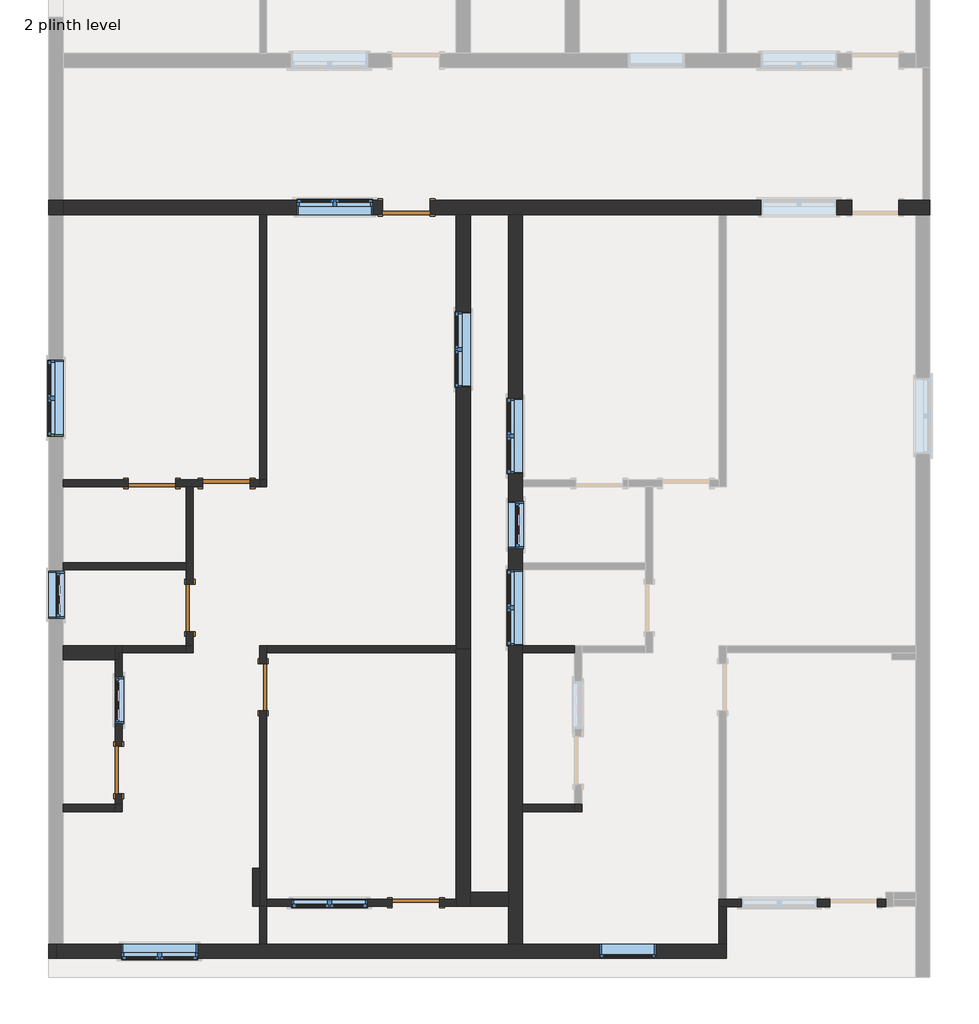
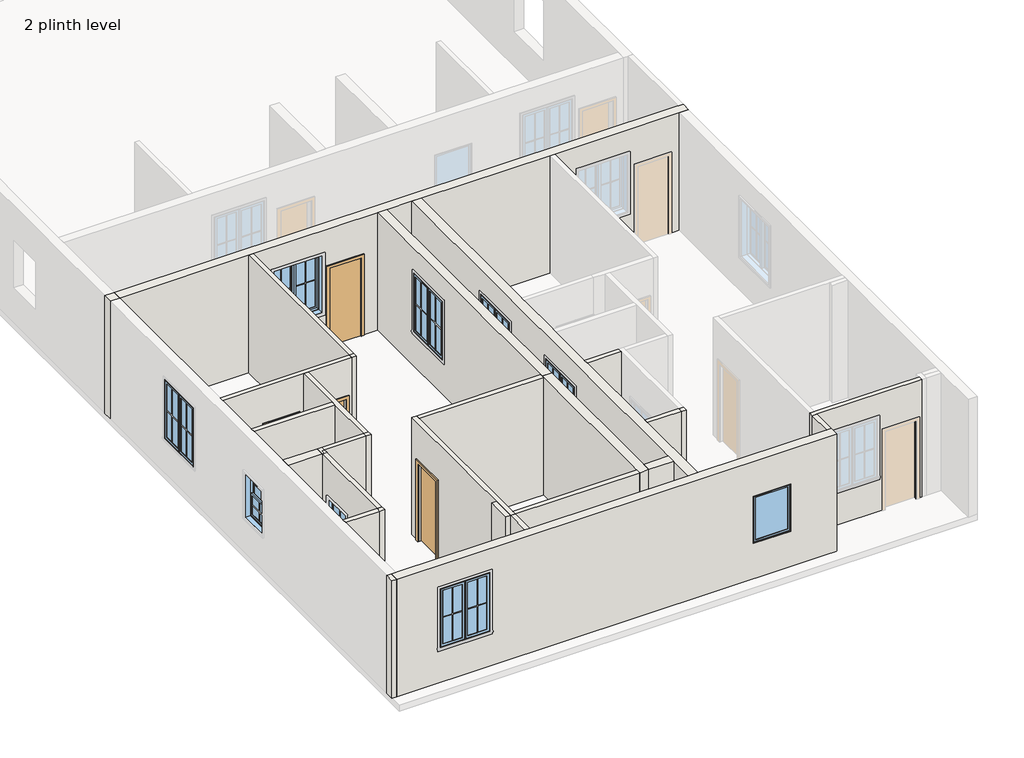
# One storey, part 1 of 4: 30 walls, 11 windows, 7 doors.
"""IFC4 building model written with IfcOpenShell, lengths in millimetres."""

from ifc_helpers import new_model, si_unit, frame, origin, place, context, project, spatial, polyline, outline, extrude, faceted_brep, transform, mapped, element, save
from components import door_d8f5dbb5, door_f2b275c1, door_85036156, window_c1f32544, window_8377141f, window_d9d3dda5, window_d400040f, window_5a369d27

model = new_model("IFC4")

# Units and contexts
model_context = context("Model", 3, world=origin())
ifc_project = project(units=[si_unit("LENGTHUNIT", "METRE", prefix="MILLI")], contexts=[model_context])

# Site, building, storey
site = spatial("IfcSite", under=ifc_project)
building = spatial("IfcBuilding", under=site)
storey = spatial("IfcBuildingStorey", under=building, Name="2 plinth level", Elevation=457.2)

# Doors
placement = place(None, origin())
door_shape = door_d8f5dbb5(model_context)
element("IfcDoor", 1, ObjectType="Single-Flush : 30\" x 80\"", at=placement, inside=storey, context=model_context, shape_type="MappedRepresentation", body=[
    mapped(door_shape, transform((-2447.3775468, -11601.0304449, 457.2), x_axis=(1.0, 0.0, 0.0), y_axis=(0.0, 1.0, 0.0), z_axis=(0.0, 0.0, 1.0))),
])
element("IfcDoor", 2, ObjectType="Single-Flush : 30\" x 80\"", at=placement, inside=storey, context=model_context, shape_type="MappedRepresentation", body=[
    mapped(door_shape, transform((-5495.3775468, -4857.3304449, 457.2), x_axis=(1.0, 0.0, 0.0), y_axis=(0.0, 1.0, 0.0), z_axis=(0.0, 0.0, 1.0))),
])
door_2_shape = door_f2b275c1(model_context)
element("IfcDoor", 3, ObjectType="Single-Flush : 30\" x 80\"", at=placement, inside=storey, context=model_context, shape_type="MappedRepresentation", body=[
    mapped(door_2_shape, transform((-4904.8275468, -8133.9304449, 457.2), x_axis=(0.0, 1.0, 0.0), y_axis=(-1.0, 0.0, 0.0), z_axis=(0.0, 0.0, 1.0))),
])
element("IfcDoor", 4, ObjectType="Single-Flush : 30\" x 80\"", at=placement, inside=storey, context=model_context, shape_type="MappedRepresentation", body=[
    mapped(door_2_shape, transform((-7228.9275468, -9467.4304449, 457.2), x_axis=(0.0, -1.0, 0.0), y_axis=(1.0, 0.0, 0.0), z_axis=(0.0, 0.0, 1.0))),
])
element("IfcDoor", 5, ObjectType="Single-Flush : 30\" x 80\"", at=placement, inside=storey, context=model_context, shape_type="MappedRepresentation", body=[
    mapped(door_2_shape, transform((-6085.9275468, -6857.5804449, 457.2), x_axis=(0.0, -1.0, 0.0), y_axis=(1.0, 0.0, 0.0), z_axis=(0.0, 0.0, 1.0))),
])
element("IfcDoor", 6, ObjectType="Single-Flush : 30\" x 80\"", at=placement, inside=storey, context=model_context, shape_type="MappedRepresentation", body=[
    mapped(door_2_shape, transform((-6695.5275468, -4857.3304449, 457.2), x_axis=(1.0, 0.0, 0.0), y_axis=(0.0, 1.0, 0.0), z_axis=(0.0, 0.0, 1.0))),
])
door_3_shape = door_85036156(model_context)
element("IfcDoor", 7, ObjectType="Single-Flush : 30\" x 80\"", at=placement, inside=storey, context=model_context, shape_type="MappedRepresentation", body=[
    mapped(door_3_shape, transform((-2599.7775468, -418.6804449, 457.2), x_axis=(1.0, 0.0, 0.0), y_axis=(0.0, 1.0, 0.0), z_axis=(0.0, 0.0, 1.0))),
])

# Walls
element("IfcWall", 8, ObjectType="4.5\"", at=placement, inside=storey, context=model_context, shape_type="Brep", body=[
    faceted_brep([(-5114.3775468, -4914.4804449, 2489.2), (-5114.3775468, -4914.4804449, 457.2), (-4961.9775468, -4914.4804449, 457.2), (-4961.9775468, -4914.4804449, 3505.2), (-6028.7775468, -4914.4804449, 3505.2), (-6143.0775468, -4914.4804449, 3505.2), (-8124.2775468, -4914.4804449, 3505.2), (-8124.2775468, -4914.4804449, 457.2), (-7076.5275468, -4914.4804449, 457.2), (-7076.5275468, -4914.4804449, 2489.2), (-6314.5275468, -4914.4804449, 2489.2), (-6314.5275468, -4914.4804449, 457.2), (-6143.0775468, -4914.4804449, 457.2), (-6028.7775468, -4914.4804449, 457.2), (-5876.3775468, -4914.4804449, 457.2), (-5876.3775468, -4914.4804449, 2489.2), (-4961.9775468, -4800.1804449, 457.2), (-5114.3775468, -4800.1804449, 457.2), (-5114.3775468, -4800.1804449, 2489.2), (-5876.3775468, -4800.1804449, 2489.2), (-5876.3775468, -4800.1804449, 457.2), (-6314.5275468, -4800.1804449, 457.2), (-6314.5275468, -4800.1804449, 2489.2), (-7076.5275468, -4800.1804449, 2489.2), (-7076.5275468, -4800.1804449, 457.2), (-8124.2775468, -4800.1804449, 457.2), (-8124.2775468, -4800.1804449, 3505.2), (-4961.9775468, -4800.1804449, 3505.2)], [[[0, 1, 2, 3, 4, 5, 6, 7, 8, 9, 10, 11, 12, 13, 14, 15]], [[16, 17, 18, 19, 20, 21, 22, 23, 24, 25, 26, 27]], [[8, 7, 25, 24]], [[2, 1, 17, 16]], [[14, 13, 12, 11, 21, 20]], [[6, 5, 4, 3, 27, 26]], [[7, 6, 26, 25]], [[3, 2, 16, 27]], [[22, 21, 11, 10]], [[23, 22, 10, 9]], [[24, 23, 9, 8]], [[18, 17, 1, 0]], [[19, 18, 0, 15]], [[20, 19, 15, 14]]]),
])
element("IfcWall", 9, ObjectType="4.5\"", at=placement, inside=storey, context=model_context, shape_type="Brep", body=[
    faceted_brep([(-6028.7775468, -7467.1804449, 457.2), (-6028.7775468, -7238.5804449, 457.2), (-6028.7775468, -7238.5804449, 2489.2), (-6028.7775468, -6476.5804449, 2489.2), (-6028.7775468, -6476.5804449, 457.2), (-6028.7775468, -4914.4804449, 457.2), (-6028.7775468, -4914.4804449, 3505.2), (-6028.7775468, -7467.1804449, 3505.2), (-6143.0775468, -7238.5804449, 2489.2), (-6143.0775468, -7238.5804449, 457.2), (-6143.0775468, -7467.1804449, 457.2), (-6143.0775468, -7467.1804449, 3505.2), (-6143.0775468, -6247.9804448, 3505.2), (-6143.0775468, -6133.6804448, 3505.2), (-6143.0775468, -4914.4804449, 3505.2), (-6143.0775468, -4914.4804449, 457.2), (-6143.0775468, -6133.6804448, 457.2), (-6143.0775468, -6247.9804448, 457.2), (-6143.0775468, -6476.5804449, 457.2), (-6143.0775468, -6476.5804449, 2489.2)], [[[0, 1, 2, 3, 4, 5, 6, 7]], [[8, 9, 10, 11, 12, 13, 14, 15, 16, 17, 18, 19]], [[10, 9, 1, 0]], [[18, 17, 16, 15, 5, 4]], [[7, 6, 14, 13, 12, 11]], [[0, 7, 11, 10]], [[6, 5, 15, 14]], [[2, 1, 9, 8]], [[3, 2, 8, 19]], [[4, 3, 19, 18]]]),
])
element("IfcWall", 10, ObjectType="4.5\"", at=placement, inside=storey, context=model_context, shape_type="SweptSolid", body=[
    extrude(outline(polyline([(-4847.6775468, -4800.1804449), (-4847.6775468, -4914.4804449), (-4961.9775468, -4914.4804449), (-4961.9775468, -4800.1804449), (-4847.6775468, -4800.1804449)])), frame((0.0, 0.0, 457.2), z_axis=(0.0, 0.0, 1.0), x_axis=(1.0, 0.0, 0.0)), (0.0, 0.0, 1.0), 3048.0),
])
element("IfcWall", 11, ObjectType="4.5\"", at=placement, inside=storey, context=model_context, shape_type="Brep", body=[
    faceted_brep([(-4847.6775468, -7752.9304449, 2489.2), (-4847.6775468, -7752.9304449, 457.2), (-4847.6775468, -7581.4804449, 457.2), (-4847.6775468, -7467.1804449, 457.2), (-4847.6775468, -7467.1804449, 3505.2), (-4847.6775468, -7581.4804449, 3505.2), (-4847.6775468, -11543.8804449, 3505.2), (-4847.6775468, -11658.1804449, 3505.2), (-4847.6775468, -11658.1804449, 457.2), (-4847.6775468, -11543.8804449, 457.2), (-4847.6775468, -8514.9304449, 457.2), (-4847.6775468, -8514.9304449, 2489.2), (-4961.9775468, -7467.1804449, 457.2), (-4961.9775468, -7752.9304449, 457.2), (-4961.9775468, -7752.9304449, 2489.2), (-4961.9775468, -8514.9304449, 2489.2), (-4961.9775468, -8514.9304449, 457.2), (-4961.9775468, -11658.1804449, 457.2), (-4961.9775468, -11658.1804449, 3505.2), (-4961.9775468, -7467.1804449, 3505.2)], [[[0, 1, 2, 3, 4, 5, 6, 7, 8, 9, 10, 11]], [[12, 13, 14, 15, 16, 17, 18, 19]], [[10, 9, 8, 17, 16]], [[3, 2, 1, 13, 12]], [[7, 6, 5, 4, 19, 18]], [[8, 7, 18, 17]], [[4, 3, 12, 19]], [[14, 13, 1, 0]], [[15, 14, 0, 11]], [[16, 15, 11, 10]]]),
])
element("IfcWall", 12, ObjectType="4.5\"", at=placement, inside=storey, context=model_context, shape_type="Brep", body=[
    faceted_brep([(-2066.3775468, -11658.1804449, 2489.2), (-2066.3775468, -11658.1804449, 457.2), (-1799.6775468, -11658.1804449, 457.2), (-1799.6775468, -11658.1804449, 3505.2), (-4847.6775468, -11658.1804449, 3505.2), (-4847.6775468, -11658.1804449, 457.2), (-2828.3775468, -11658.1804449, 457.2), (-2828.3775468, -11658.1804449, 2489.2), (-4447.6275468, -11658.1804449, 2895.6), (-3228.4275468, -11658.1804449, 2895.6), (-3228.4275468, -11658.1804449, 1371.6), (-4447.6275468, -11658.1804449, 1371.6), (-1799.6775468, -11543.8804449, 457.2), (-2066.3775468, -11543.8804449, 457.2), (-2066.3775468, -11543.8804449, 2489.2), (-2828.3775468, -11543.8804449, 2489.2), (-2828.3775468, -11543.8804449, 457.2), (-4847.6775468, -11543.8804449, 457.2), (-4847.6775468, -11543.8804449, 3505.2), (-1799.6775468, -11543.8804449, 3505.2), (-4447.6275468, -11543.8804449, 2895.6), (-4447.6275468, -11543.8804449, 1371.6), (-3228.4275468, -11543.8804449, 1371.6), (-3228.4275468, -11543.8804449, 2895.6), (-1799.6775468, -11657.3545138, 457.2), (-1799.6775468, -11657.3545138, 3505.2)], [[[0, 1, 2, 3, 4, 5, 6, 7], [8, 9, 10, 11]], [[12, 13, 14, 15, 16, 17, 18, 19], [20, 21, 22, 23]], [[6, 5, 17, 16]], [[2, 1, 13, 12, 24]], [[4, 3, 25, 19, 18]], [[5, 4, 18, 17]], [[3, 2, 24, 12, 19, 25]], [[14, 13, 1, 0]], [[15, 14, 0, 7]], [[16, 15, 7, 6]], [[21, 20, 8, 11]], [[22, 21, 11, 10]], [[23, 22, 10, 9]], [[20, 23, 9, 8]]]),
])
element("IfcWall", 13, ObjectType="4.5\"", at=placement, inside=storey, context=model_context, shape_type="SweptSolid", body=[
    extrude(outline(polyline([(-7171.7775468, -10134.1804449), (-7286.0775468, -10134.1804449), (-7286.0775468, -10019.8804449), (-7171.7775468, -10019.8804449), (-7171.7775468, -10134.1804449)])), frame((0.0, 0.0, 457.2), z_axis=(0.0, 0.0, 1.0), x_axis=(1.0, 0.0, 0.0)), (0.0, 0.0, 1.0), 3048.0),
])
element("IfcWall", 14, ObjectType="4.5\"", at=placement, inside=storey, context=model_context, shape_type="Brep", body=[
    faceted_brep([(-7286.0775468, -7467.1804449, 457.2), (-7286.0775468, -7695.7804449, 457.2), (-7286.0775468, -7695.7804449, 3505.2), (-7286.0775468, -7467.1804449, 3505.2), (-7171.7775468, -7467.1804449, 457.2), (-7171.7775468, -7467.1804449, 3505.2), (-7171.7775468, -7581.4804449, 3505.2), (-7171.7775468, -7695.7804449, 3505.2), (-7171.7775468, -7695.7804449, 457.2), (-7171.7775468, -7581.4804449, 457.2)], [[[0, 1, 2, 3]], [[4, 5, 6, 7, 8, 9]], [[1, 0, 4, 9, 8]], [[2, 1, 8, 7]], [[3, 2, 7, 6, 5]], [[0, 3, 5, 4]]]),
])
element("IfcWall", 15, ObjectType="4.5\"", at=placement, inside=storey, context=model_context, shape_type="SweptSolid", body=[
    extrude(outline(polyline([(-8124.2775468, -6133.6804448), (-6143.0775468, -6133.6804448), (-6143.0775468, -6247.9804448), (-8124.2775468, -6247.9804448), (-8124.2775468, -6133.6804448)])), frame((0.0, 0.0, 457.2), z_axis=(0.0, 0.0, 1.0), x_axis=(1.0, 0.0, 0.0)), (0.0, 0.0, 1.0), 3048.0),
])
element("IfcWall", 16, ObjectType="4.5\"", at=placement, inside=storey, context=model_context, shape_type="Brep", body=[
    faceted_brep([(-7171.7775468, -10019.8804449, 457.2), (-7171.7775468, -9848.4304449, 457.2), (-7171.7775468, -9848.4304449, 2489.2), (-7171.7775468, -9086.4304449, 2489.2), (-7171.7775468, -9086.4304449, 457.2), (-7171.7775468, -7581.4804449, 457.2), (-7171.7775468, -7581.4804449, 3505.2), (-7171.7775468, -10019.8804449, 3505.2), (-7171.7775468, -7962.4804449, 2540.0), (-7171.7775468, -7962.4804449, 1371.6), (-7171.7775468, -8724.4804449, 1371.6), (-7171.7775468, -8724.4804449, 2540.0), (-7286.0775468, -9848.4304449, 2489.2), (-7286.0775468, -9848.4304449, 457.2), (-7286.0775468, -10019.8804449, 457.2), (-7286.0775468, -10019.8804449, 3505.2), (-7286.0775468, -7695.7804449, 3505.2), (-7286.0775468, -7695.7804449, 457.2), (-7286.0775468, -9086.4304449, 457.2), (-7286.0775468, -9086.4304449, 2489.2), (-7286.0775468, -7962.4804449, 2540.0), (-7286.0775468, -8724.4804449, 2540.0), (-7286.0775468, -8724.4804449, 1371.6), (-7286.0775468, -7962.4804449, 1371.6), (-7228.9275468, -7695.7804449, 457.2), (-7228.9275468, -7581.4804449, 457.2), (-7228.9275468, -7581.4804449, 3505.2), (-7228.9275468, -7695.7804449, 3505.2)], [[[0, 1, 2, 3, 4, 5, 6, 7], [8, 9, 10, 11]], [[12, 13, 14, 15, 16, 17, 18, 19], [20, 21, 22, 23]], [[18, 17, 24, 25, 5, 4]], [[14, 13, 1, 0]], [[7, 6, 26, 27, 16, 15]], [[6, 5, 25, 26]], [[25, 24, 27, 26]], [[24, 17, 16, 27]], [[0, 7, 15, 14]], [[2, 1, 13, 12]], [[3, 2, 12, 19]], [[4, 3, 19, 18]], [[9, 8, 20, 23]], [[10, 9, 23, 22]], [[11, 10, 22, 21]], [[8, 11, 21, 20]]]),
])
element("IfcWall", 17, ObjectType="4.5\"", at=placement, inside=storey, context=model_context, shape_type="SweptSolid", body=[
    extrude(outline(polyline([(-6028.7775468, -7581.4804449), (-6143.0775468, -7581.4804449), (-6143.0775468, -7467.1804449), (-6028.7775468, -7467.1804449), (-6028.7775468, -7581.4804449)])), frame((0.0, 0.0, 457.2), z_axis=(0.0, 0.0, 1.0), x_axis=(1.0, 0.0, 0.0)), (0.0, 0.0, 1.0), 3048.0),
])
element("IfcWall", 18, ObjectType="4.5\"", at=placement, inside=storey, context=model_context, shape_type="SweptSolid", body=[
    extrude(outline(polyline([(-4961.9775468, -12267.7804449), (-4961.9775468, -11658.1804449), (-4847.6775468, -11658.1804449), (-4847.6775468, -12267.7804449), (-4961.9775468, -12267.7804449)])), frame((0.0, 0.0, 457.2), z_axis=(0.0, 0.0, 1.0), x_axis=(1.0, 0.0, 0.0)), (0.0, 0.0, 1.0), 3048.0),
])
element("IfcWall", 19, ObjectType="4.5\"", at=placement, inside=storey, context=model_context, shape_type="Brep", body=[
    faceted_brep([(5114.9115487, -11546.9284449, 457.2), (4971.996455, -11546.9284449, 457.2), (4971.996455, -11546.9284449, 2489.2), (4209.996455, -11546.9284449, 2489.2), (4209.996455, -11546.9284449, 457.2), (4067.0813613, -11546.9284449, 457.2), (3952.7813613, -11546.9284449, 457.2), (2543.7224532, -11546.9284449, 457.2), (2429.4224532, -11546.9284449, 457.2), (2429.4224532, -11546.9284449, 3505.2), (2543.7224532, -11546.9284449, 3505.2), (3952.7813613, -11546.9284449, 3505.2), (4067.0813613, -11546.9284449, 3505.2), (5114.9115487, -11546.9284449, 3505.2), (2790.7313613, -11546.9284449, 2895.6), (2790.7313613, -11546.9284449, 1371.6), (4009.9313613, -11546.9284449, 1371.6), (4009.9313613, -11546.9284449, 2895.6), (4971.996455, -11661.2284449, 2489.2), (4971.996455, -11661.2284449, 457.2), (5114.9115487, -11661.2284449, 457.2), (5114.9115487, -11661.2284449, 3505.2), (2543.7224532, -11661.2284449, 3505.2), (2429.4224532, -11661.2284449, 3505.2), (2429.4224532, -11661.2284449, 457.2), (2543.7224532, -11661.2284449, 457.2), (4209.996455, -11661.2284449, 457.2), (4209.996455, -11661.2284449, 2489.2), (2790.7313613, -11661.2284449, 2895.6), (4009.9313613, -11661.2284449, 2895.6), (4009.9313613, -11661.2284449, 1371.6), (2790.7313613, -11661.2284449, 1371.6)], [[[0, 1, 2, 3, 4, 5, 6, 7, 8, 9, 10, 11, 12, 13], [14, 15, 16, 17]], [[18, 19, 20, 21, 22, 23, 24, 25, 26, 27], [28, 29, 30, 31]], [[20, 19, 1, 0]], [[26, 25, 24, 8, 7, 6, 5, 4]], [[13, 12, 11, 10, 9, 23, 22, 21]], [[9, 8, 24, 23]], [[0, 13, 21, 20]], [[2, 1, 19, 18]], [[3, 2, 18, 27]], [[4, 3, 27, 26]], [[15, 14, 28, 31]], [[16, 15, 31, 30]], [[17, 16, 30, 29]], [[14, 17, 29, 28]]]),
])
element("IfcWall", 20, ObjectType="4.5\"", at=placement, inside=storey, context=model_context, shape_type="Brep", body=[
    faceted_brep([(-4847.6775468, -7581.4804449, 457.2), (-1799.6775468, -7581.4804449, 457.2), (-1799.6775468, -7581.4804449, 3505.2), (-4847.6775468, -7581.4804449, 3505.2), (-4847.6775468, -7467.1804449, 457.2), (-4847.6775468, -7467.1804449, 3505.2), (-1799.6775468, -7467.1804449, 3505.2), (-1799.6775468, -7467.1804449, 457.2), (-1799.6775468, -7524.3304449, 457.2), (-1799.6775468, -7524.3304449, 3505.2)], [[[0, 1, 2, 3]], [[4, 5, 6, 7]], [[1, 0, 4, 7, 8]], [[3, 2, 9, 6, 5]], [[2, 1, 8, 7, 6, 9]], [[0, 3, 5, 4]]]),
])
element("IfcWall", 21, ObjectType="4.5\"", at=placement, inside=storey, context=model_context, shape_type="SweptSolid", body=[
    extrude(outline(polyline([(-4847.6775468, -532.9804449), (-4847.6775468, -4800.1804449), (-4961.9775468, -4800.1804449), (-4961.9775468, -532.9804449), (-4847.6775468, -532.9804449)])), frame((0.0, 0.0, 457.2), z_axis=(0.0, 0.0, 1.0), x_axis=(1.0, 0.0, 0.0)), (0.0, 0.0, 1.0), 3048.0),
])
element("IfcWall", 22, ObjectType="4.5\"", at=placement, inside=storey, context=model_context, shape_type="SweptSolid", body=[
    extrude(outline(polyline([(-6143.0775468, -7581.4804449), (-7171.7775468, -7581.4804449), (-7171.7775468, -7467.1804449), (-6143.0775468, -7467.1804449), (-6143.0775468, -7581.4804449)])), frame((0.0, 0.0, 457.2), z_axis=(0.0, 0.0, 1.0), x_axis=(1.0, 0.0, 0.0)), (0.0, 0.0, 1.0), 3048.0),
])
element("IfcWall", 23, ObjectType="4.5\"", at=placement, inside=storey, context=model_context, shape_type="SweptSolid", body=[
    extrude(outline(polyline([(-7286.0775468, -10134.1804449), (-8124.2775468, -10134.1804449), (-8124.2775468, -10019.8804449), (-7286.0775468, -10019.8804449), (-7286.0775468, -10134.1804449)])), frame((0.0, 0.0, 457.2), z_axis=(0.0, 0.0, 1.0), x_axis=(1.0, 0.0, 0.0)), (0.0, 0.0, 1.0), 3048.0),
])
element("IfcWall", 24, ObjectType="4.5\"", at=placement, inside=storey, context=model_context, shape_type="SweptSolid", body=[
    extrude(outline(polyline([(105.3224532, -10134.1804449), (-732.8775468, -10134.1804449), (-732.8775468, -10019.8804449), (105.3224532, -10019.8804449), (105.3224532, -10134.1804449)])), frame((0.0, 0.0, 457.2), z_axis=(0.0, 0.0, 1.0), x_axis=(1.0, 0.0, 0.0)), (0.0, 0.0, 1.0), 3048.0),
])
element("IfcWall", 25, ObjectType="4.5\"", at=placement, inside=storey, context=model_context, shape_type="SweptSolid", body=[
    extrude(outline(polyline([(2543.7224532, -11661.2284449), (2543.7224532, -12267.7804449), (2429.4224532, -12267.7804449), (2429.4224532, -11661.2284449), (2543.7224532, -11661.2284449)])), frame((0.0, 0.0, 457.2), z_axis=(0.0, 0.0, 1.0), x_axis=(1.0, 0.0, 0.0)), (0.0, 0.0, 1.0), 3048.0),
])
element("IfcWall", 26, ObjectType="4.5\"", at=placement, inside=storey, context=model_context, shape_type="SweptSolid", body=[
    extrude(outline(polyline([(219.6224532, -10019.8804449), (219.6224532, -10134.1804449), (105.3224532, -10134.1804449), (105.3224532, -10019.8804449), (219.6224532, -10019.8804449)])), frame((0.0, 0.0, 457.2), z_axis=(0.0, 0.0, 1.0), x_axis=(1.0, 0.0, 0.0)), (0.0, 0.0, 1.0), 3048.0),
])
element("IfcWall", 27, ObjectType="4.5\"", at=placement, inside=storey, context=model_context, shape_type="SweptSolid", body=[
    extrude(outline(polyline([(105.3224532, -7581.4804449), (-732.8775468, -7581.4804449), (-732.8775468, -7467.1804449), (105.3224532, -7467.1804449), (105.3224532, -7581.4804449)])), frame((0.0, 0.0, 457.2), z_axis=(0.0, 0.0, 1.0), x_axis=(1.0, 0.0, 0.0)), (0.0, 0.0, 1.0), 3048.0),
])
element("IfcWall", 28, ObjectType="4.5\"", at=placement, inside=storey, context=model_context, shape_type="SweptSolid", body=[
    extrude(outline(polyline([(-5076.2775468, -11658.1804449), (-5076.2775468, -11048.5804449), (-4961.9775468, -11048.5804449), (-4961.9775468, -11658.1804449), (-5076.2775468, -11658.1804449)])), frame((0.0, 0.0, 457.2), z_axis=(0.0, 0.0, 1.0), x_axis=(1.0, 0.0, 0.0)), (0.0, 0.0, 1.0), 3048.0),
])
element("IfcWall", 29, ObjectType="9\"", at=placement, inside=storey, context=model_context, shape_type="Brep", body=[
    faceted_brep([(2543.7224532, -12267.7804449, 457.2), (2429.4224532, -12267.7804449, 457.2), (-732.8775468, -12267.7804449, 457.2), (-961.4775468, -12267.7804449, 457.2), (-4847.6775468, -12267.7804449, 457.2), (-4961.9775468, -12267.7804449, 457.2), (-8124.2775468, -12267.7804449, 457.2), (-8238.5775468, -12267.7804449, 457.2), (-8238.5775468, -12267.7804449, 3505.2), (-8124.2775468, -12267.7804449, 3505.2), (-4961.9775468, -12267.7804449, 3505.2), (-4847.6775468, -12267.7804449, 3505.2), (-961.4775468, -12267.7804449, 3505.2), (-732.8775468, -12267.7804449, 3505.2), (2429.4224532, -12267.7804449, 3505.2), (2543.7224532, -12267.7804449, 3505.2), (505.3724532, -12267.7804449, 2590.8), (505.3724532, -12267.7804449, 1371.6), (1419.7724532, -12267.7804449, 1371.6), (1419.7724532, -12267.7804449, 2590.8), (-7181.3025468, -12267.7804449, 2895.6), (-7181.3025468, -12267.7804449, 1371.6), (-5962.1025468, -12267.7804449, 1371.6), (-5962.1025468, -12267.7804449, 2895.6), (2543.7224532, -12496.3804449, 457.2), (2543.7224532, -12496.3804449, 3505.2), (-8238.5775468, -12496.3804449, 3505.2), (-8238.5775468, -12496.3804449, 457.2), (505.3724532, -12496.3804449, 2590.8), (1419.7724532, -12496.3804449, 2590.8), (1419.7724532, -12496.3804449, 1371.6), (505.3724532, -12496.3804449, 1371.6), (-7181.3025468, -12496.3804449, 2895.6), (-5962.1025468, -12496.3804449, 2895.6), (-5962.1025468, -12496.3804449, 1371.6), (-7181.3025468, -12496.3804449, 1371.6)], [[[0, 1, 2, 3, 4, 5, 6, 7, 8, 9, 10, 11, 12, 13, 14, 15], [16, 17, 18, 19], [20, 21, 22, 23]], [[24, 25, 26, 27], [28, 29, 30, 31], [32, 33, 34, 35]], [[7, 6, 5, 4, 3, 2, 1, 0, 24, 27]], [[8, 7, 27, 26]], [[15, 14, 13, 12, 11, 10, 9, 8, 26, 25]], [[0, 15, 25, 24]], [[17, 16, 28, 31]], [[18, 17, 31, 30]], [[19, 18, 30, 29]], [[16, 19, 29, 28]], [[21, 20, 32, 35]], [[22, 21, 35, 34]], [[23, 22, 34, 33]], [[20, 23, 33, 32]]]),
])
element("IfcWall", 30, ObjectType="9\"", at=placement, inside=storey, context=model_context, shape_type="Brep", body=[
    faceted_brep([(-1571.0775468, -11658.1804449, 457.2), (-1571.0775468, -11429.5789528, 457.2), (-1571.0775468, -7524.3304449, 457.2), (-1571.0775468, -7524.3304449, 3505.2), (-1571.0775468, -11429.5789528, 3505.2), (-1571.0775468, -11658.1804449, 3505.2), (-1799.6775468, -11657.3545138, 457.2), (-1799.6775468, -11657.3545138, 3505.2), (-1799.6775468, -11543.8804449, 3505.2), (-1799.6775468, -7581.4804449, 3505.2), (-1799.6775468, -7524.3304449, 3505.2), (-1799.6775468, -7524.3304449, 457.2), (-1799.6775468, -7581.4804449, 457.2), (-1799.6775468, -11543.8804449, 457.2)], [[[0, 1, 2, 3, 4, 5]], [[6, 7, 8, 9, 10, 11, 12, 13]], [[2, 1, 0, 6, 13, 12, 11]], [[3, 2, 11, 10]], [[5, 4, 3, 10, 9, 8, 7]], [[0, 5, 7, 6]]]),
])
element("IfcWall", 31, ObjectType="9\"", at=placement, inside=storey, context=model_context, shape_type="SweptSolid", body=[
    extrude(outline(polyline([(-8352.8775468, -532.9804449), (-8352.8775468, -304.3804449), (-8124.2775468, -304.3804449), (-8124.2775468, -532.9804449), (-8352.8775468, -532.9804449)])), frame((0.0, 0.0, 457.2), z_axis=(0.0, 0.0, 1.0), x_axis=(1.0, 0.0, 0.0)), (0.0, 0.0, 1.0), 3048.0),
])
element("IfcWall", 32, ObjectType="9\"", at=placement, inside=storey, context=model_context, shape_type="Brep", body=[
    faceted_brep([(5820.3224532, -304.3804449, 457.2), (5706.0224532, -304.3804449, 457.2), (5325.0224532, -304.3804449, 457.2), (5325.0224532, -304.3804449, 2489.2), (4563.0224532, -304.3804449, 2489.2), (4563.0224532, -304.3804449, 457.2), (-2218.7775468, -304.3804449, 457.2), (-2218.7775468, -304.3804449, 2489.2), (-2980.7775468, -304.3804449, 2489.2), (-2980.7775468, -304.3804449, 457.2), (-8124.2775468, -304.3804449, 457.2), (-8124.2775468, -304.3804449, 3505.2), (5706.0224532, -304.3804449, 3505.2), (5820.3224532, -304.3804449, 3505.2), (-3142.7025468, -304.3804449, 2895.6), (-4361.9025468, -304.3804449, 2895.6), (-4361.9025468, -304.3804449, 1371.6), (-3142.7025468, -304.3804449, 1371.6), (4324.8974532, -304.3804449, 2895.6), (3105.6974532, -304.3804449, 2895.6), (3105.6974532, -304.3804449, 1371.6), (4324.8974532, -304.3804449, 1371.6), (5325.0224532, -532.9804449, 2489.2), (5325.0224532, -532.9804449, 457.2), (5591.7224532, -532.9804449, 457.2), (5820.3224532, -532.9804449, 457.2), (5820.3224532, -532.9804449, 3505.2), (5591.7224532, -532.9804449, 3505.2), (2543.7224532, -532.9804449, 3505.2), (2429.4224532, -532.9804449, 3505.2), (-732.8775468, -532.9804449, 3505.2), (-961.4775468, -532.9804449, 3505.2), (-1571.0775468, -532.9804449, 3505.2), (-1799.6775468, -532.9804449, 3505.2), (-4847.6775468, -532.9804449, 3505.2), (-4961.9775468, -532.9804449, 3505.2), (-8124.2775468, -532.9804449, 3505.2), (-8124.2775468, -532.9804449, 457.2), (-4961.9775468, -532.9804449, 457.2), (-4847.6775468, -532.9804449, 457.2), (-2980.7775468, -532.9804449, 457.2), (-2980.7775468, -532.9804449, 2489.2), (-2218.7775468, -532.9804449, 2489.2), (-2218.7775468, -532.9804449, 457.2), (-1799.6775468, -532.9804449, 457.2), (-1571.0775468, -532.9804449, 457.2), (-961.4775468, -532.9804449, 457.2), (-732.8775468, -532.9804449, 457.2), (2429.4224532, -532.9804449, 457.2), (2543.7224532, -532.9804449, 457.2), (4563.0224532, -532.9804449, 457.2), (4563.0224532, -532.9804449, 2489.2), (-3142.7025468, -532.9804449, 2895.6), (-3142.7025468, -532.9804449, 1371.6), (-4361.9025468, -532.9804449, 1371.6), (-4361.9025468, -532.9804449, 2895.6), (4324.8974532, -532.9804449, 2895.6), (4324.8974532, -532.9804449, 1371.6), (3105.6974532, -532.9804449, 1371.6), (3105.6974532, -532.9804449, 2895.6)], [[[0, 1, 2, 3, 4, 5, 6, 7, 8, 9, 10, 11, 12, 13], [14, 15, 16, 17], [18, 19, 20, 21]], [[22, 23, 24, 25, 26, 27, 28, 29, 30, 31, 32, 33, 34, 35, 36, 37, 38, 39, 40, 41, 42, 43, 44, 45, 46, 47, 48, 49, 50, 51], [52, 53, 54, 55], [56, 57, 58, 59]], [[40, 39, 38, 37, 10, 9]], [[25, 24, 23, 2, 1, 0]], [[50, 49, 48, 47, 46, 45, 44, 43, 6, 5]], [[13, 12, 11, 36, 35, 34, 33, 32, 31, 30, 29, 28, 27, 26]], [[11, 10, 37, 36]], [[0, 13, 26, 25]], [[7, 6, 43, 42]], [[8, 7, 42, 41]], [[9, 8, 41, 40]], [[3, 2, 23, 22]], [[4, 3, 22, 51]], [[5, 4, 51, 50]], [[53, 52, 14, 17]], [[54, 53, 17, 16]], [[55, 54, 16, 15]], [[52, 55, 15, 14]], [[57, 56, 18, 21]], [[58, 57, 21, 20]], [[59, 58, 20, 19]], [[56, 59, 19, 18]]]),
])
element("IfcWall", 33, ObjectType="9\"", at=placement, inside=storey, context=model_context, shape_type="SweptSolid", body=[
    extrude(outline(polyline([(-8352.8775468, -12267.7804449), (-8238.5775468, -12267.7804449), (-8238.5775468, -12496.3804449), (-8352.8775468, -12496.3804449), (-8352.8775468, -12267.7804449)])), frame((0.0, 0.0, 457.2), z_axis=(0.0, 0.0, 1.0), x_axis=(1.0, 0.0, 0.0)), (0.0, 0.0, 1.0), 3048.0),
])
element("IfcWall", 34, ObjectType="9\"", at=placement, inside=storey, context=model_context, shape_type="Brep", body=[
    faceted_brep([(-961.4775468, -532.9804449, 457.2), (-961.4775468, -11431.7814356, 457.2), (-961.4775468, -11660.3829276, 457.2), (-961.4775468, -12267.7804449, 457.2), (-961.4775468, -12267.7804449, 3505.2), (-961.4775468, -11660.3829276, 3505.2), (-961.4775468, -11431.7814356, 3505.2), (-961.4775468, -532.9804449, 3505.2), (-961.4775468, -3485.7304449, 2895.6), (-961.4775468, -4704.9304449, 2895.6), (-961.4775468, -4704.9304449, 1371.6), (-961.4775468, -3485.7304449, 1371.6), (-961.4775468, -6247.9804449, 2895.6), (-961.4775468, -7467.1804449, 2895.6), (-961.4775468, -7467.1804449, 1371.6), (-961.4775468, -6247.9804449, 1371.6), (-961.4775468, -5143.0804449, 2540.0), (-961.4775468, -5905.0804449, 2540.0), (-961.4775468, -5905.0804449, 1371.6), (-961.4775468, -5143.0804449, 1371.6), (-732.8775468, -532.9804449, 457.2), (-732.8775468, -532.9804449, 3505.2), (-732.8775468, -4800.1804449, 3505.2), (-732.8775468, -4914.4804449, 3505.2), (-732.8775468, -6133.6804449, 3505.2), (-732.8775468, -6247.9804449, 3505.2), (-732.8775468, -7467.1804449, 3505.2), (-732.8775468, -7581.4804449, 3505.2), (-732.8775468, -10019.8804449, 3505.2), (-732.8775468, -10134.1804449, 3505.2), (-732.8775468, -12267.7804449, 3505.2), (-732.8775468, -12267.7804449, 457.2), (-732.8775468, -10134.1804449, 457.2), (-732.8775468, -10019.8804449, 457.2), (-732.8775468, -7581.4804449, 457.2), (-732.8775468, -7467.1804449, 457.2), (-732.8775468, -6247.9804449, 457.2), (-732.8775468, -6133.6804449, 457.2), (-732.8775468, -4914.4804449, 457.2), (-732.8775468, -4800.1804449, 457.2), (-732.8775468, -3485.7304449, 2895.6), (-732.8775468, -3485.7304449, 1371.6), (-732.8775468, -4704.9304449, 1371.6), (-732.8775468, -4704.9304449, 2895.6), (-732.8775468, -6247.9804449, 2895.6), (-732.8775468, -6247.9804449, 1371.6), (-732.8775468, -7467.1804449, 1371.6), (-732.8775468, -7467.1804449, 2895.6), (-732.8775468, -5143.0804449, 2540.0), (-732.8775468, -5143.0804449, 1371.6), (-732.8775468, -5905.0804449, 1371.6), (-732.8775468, -5905.0804449, 2540.0)], [[[0, 1, 2, 3, 4, 5, 6, 7], [8, 9, 10, 11], [12, 13, 14, 15], [16, 17, 18, 19]], [[20, 21, 22, 23, 24, 25, 26, 27, 28, 29, 30, 31, 32, 33, 34, 35, 36, 37, 38, 39], [40, 41, 42, 43], [44, 45, 46, 47], [48, 49, 50, 51]], [[3, 2, 1, 0, 20, 39, 38, 37, 36, 35, 34, 33, 32, 31]], [[7, 6, 5, 4, 30, 29, 28, 27, 26, 25, 24, 23, 22, 21]], [[0, 7, 21, 20]], [[4, 3, 31, 30]], [[41, 40, 8, 11]], [[42, 41, 11, 10]], [[43, 42, 10, 9]], [[40, 43, 9, 8]], [[45, 44, 12, 15]], [[46, 45, 15, 14]], [[47, 46, 14, 13]], [[44, 47, 13, 12]], [[49, 48, 16, 19]], [[50, 49, 19, 18]], [[51, 50, 18, 17]], [[48, 51, 17, 16]]]),
])
element("IfcWall", 35, ObjectType="9\"", at=placement, inside=storey, context=model_context, shape_type="Brep", body=[
    faceted_brep([(-1571.0775468, -7524.3304449, 457.2), (-1571.0775468, -532.9804449, 457.2), (-1571.0775468, -532.9804449, 3505.2), (-1571.0775468, -7524.3304449, 3505.2), (-1571.0775468, -2095.0804449, 2895.6), (-1571.0775468, -2095.0804449, 1371.6), (-1571.0775468, -3314.2804449, 1371.6), (-1571.0775468, -3314.2804449, 2895.6), (-1799.6775468, -7524.3304449, 457.2), (-1799.6775468, -7524.3304449, 3505.2), (-1799.6775468, -7467.1804449, 3505.2), (-1799.6775468, -532.9804449, 3505.2), (-1799.6775468, -532.9804449, 457.2), (-1799.6775468, -7467.1804449, 457.2), (-1799.6775468, -2095.0804449, 2895.6), (-1799.6775468, -3314.2804449, 2895.6), (-1799.6775468, -3314.2804449, 1371.6), (-1799.6775468, -2095.0804449, 1371.6)], [[[0, 1, 2, 3], [4, 5, 6, 7]], [[8, 9, 10, 11, 12, 13], [14, 15, 16, 17]], [[1, 0, 8, 13, 12]], [[3, 2, 11, 10, 9]], [[0, 3, 9, 8]], [[2, 1, 12, 11]], [[5, 4, 14, 17]], [[6, 5, 17, 16]], [[7, 6, 16, 15]], [[4, 7, 15, 14]]]),
])
element("IfcWall", 36, ObjectType="9\"", at=placement, inside=storey, context=model_context, shape_type="SweptSolid", body=[
    extrude(outline(polyline([(-7286.0775468, -7695.7804449), (-8124.2775468, -7695.7804449), (-8124.2775468, -7467.1804449), (-7286.0775468, -7467.1804449), (-7286.0775468, -7695.7804449)])), frame((0.0, 0.0, 457.2), z_axis=(0.0, 0.0, 1.0), x_axis=(1.0, 0.0, 0.0)), (0.0, 0.0, 1.0), 3048.0),
])
element("IfcWall", 37, ObjectType="9\"", at=placement, inside=storey, context=model_context, shape_type="SweptSolid", body=[
    extrude(outline(polyline([(-1571.0775468, -11429.5789528), (-961.4775468, -11431.7814356), (-961.4775468, -11660.3829276), (-1571.0775468, -11658.1804449), (-1571.0775468, -11429.5789528)])), frame((0.0, 0.0, 457.2), z_axis=(0.0, 0.0, 1.0), x_axis=(1.0, 0.0, 0.0)), (0.0, 0.0, 1.0), 3048.0),
])

# Windows
window_shape = window_c1f32544(model_context)
element("IfcWindow", 38, ObjectType="Fixed : 36\" x 48\"", at=placement, inside=storey, context=model_context, shape_type="MappedRepresentation", body=[
    mapped(window_shape, transform((924.4724532, -12382.0804449, 457.2), x_axis=(-1.0, 0.0, 0.0), y_axis=(0.0, -1.0, 0.0), z_axis=(0.0, 0.0, 1.0))),
])
window_2_shape = window_8377141f(model_context)
element("IfcWindow", 39, ObjectType="Window-Casement-Double : 48\" x 60\"", at=placement, inside=storey, context=model_context, shape_type="MappedRepresentation", body=[
    mapped(window_2_shape, transform((-8238.5775468, -3485.7304449, 457.2), x_axis=(0.0, 1.0, 0.0), y_axis=(-1.0, 0.0, 0.0), z_axis=(0.0, 0.0, 1.0))),
])
element("IfcWindow", 40, ObjectType="Window-Casement-Double : 48\" x 60\"", at=placement, inside=storey, context=model_context, shape_type="MappedRepresentation", body=[
    mapped(window_2_shape, transform((-3752.3025468, -418.6804449, 457.2), x_axis=(1.0, 0.0, 0.0), y_axis=(0.0, 1.0, 0.0), z_axis=(0.0, 0.0, 1.0))),
])
element("IfcWindow", 41, ObjectType="Window-Casement-Double : 48\" x 60\"", at=placement, inside=storey, context=model_context, shape_type="MappedRepresentation", body=[
    mapped(window_2_shape, transform((-1685.3775468, -2704.6804449, 457.2), x_axis=(0.0, 1.0, 0.0), y_axis=(-1.0, 0.0, 0.0), z_axis=(0.0, 0.0, 1.0))),
])
element("IfcWindow", 42, ObjectType="Window-Casement-Double : 48\" x 60\"", at=placement, inside=storey, context=model_context, shape_type="MappedRepresentation", body=[
    mapped(window_2_shape, transform((-847.1775468, -4095.3304449, 457.2), x_axis=(0.0, 1.0, 0.0), y_axis=(-1.0, 0.0, 0.0), z_axis=(0.0, 0.0, 1.0))),
])
element("IfcWindow", 43, ObjectType="Window-Casement-Double : 48\" x 60\"", at=placement, inside=storey, context=model_context, shape_type="MappedRepresentation", body=[
    mapped(window_2_shape, transform((-847.1775468, -6857.5804449, 457.2), x_axis=(0.0, 1.0, 0.0), y_axis=(-1.0, 0.0, 0.0), z_axis=(0.0, 0.0, 1.0))),
])
element("IfcWindow", 44, ObjectType="Window-Casement-Double : 48\" x 60\"", at=placement, inside=storey, context=model_context, shape_type="MappedRepresentation", body=[
    mapped(window_2_shape, transform((-6571.7025468, -12382.0804449, 457.2), x_axis=(-1.0, 0.0, 0.0), y_axis=(0.0, -1.0, 0.0), z_axis=(0.0, 0.0, 1.0))),
])
window_3_shape = window_d9d3dda5(model_context)
element("IfcWindow", 45, ObjectType="Window-Casement-Double : 48\" x 60\"", at=placement, inside=storey, context=model_context, shape_type="MappedRepresentation", body=[
    mapped(window_3_shape, transform((-3838.0275468, -11601.0304449, 457.2), x_axis=(-1.0, 0.0, 0.0), y_axis=(0.0, -1.0, 0.0), z_axis=(0.0, 0.0, 1.0))),
])
window_4_shape = window_d400040f(model_context)
element("IfcWindow", 46, ObjectType="Window-Double-Hung : 30\" x 46\"", at=placement, inside=storey, context=model_context, shape_type="MappedRepresentation", body=[
    mapped(window_4_shape, transform((-8238.5775468, -6648.0304448, 457.2), x_axis=(0.0, -1.0, 0.0), y_axis=(1.0, 0.0, 0.0), z_axis=(0.0, 0.0, 1.0))),
])
element("IfcWindow", 47, ObjectType="Window-Double-Hung : 30\" x 46\"", at=placement, inside=storey, context=model_context, shape_type="MappedRepresentation", body=[
    mapped(window_4_shape, transform((-847.1775468, -5524.0804449, 457.2), x_axis=(0.0, -1.0, 0.0), y_axis=(1.0, 0.0, 0.0), z_axis=(0.0, 0.0, 1.0))),
])
window_5_shape = window_5a369d27(model_context)
element("IfcWindow", 48, ObjectType="Window-Double-Hung : 30\" x 46\"", at=placement, inside=storey, context=model_context, shape_type="MappedRepresentation", body=[
    mapped(window_5_shape, transform((-7228.9275468, -8343.4804449, 457.2), x_axis=(0.0, -1.0, 0.0), y_axis=(1.0, 0.0, 0.0), z_axis=(0.0, 0.0, 1.0))),
])

save(model, "model.ifc")

# Revit data of these elements
# Type "Single-Flush : 30\" x 80\""
#   Type Mark = "5"
#   Construction Type Id = "MDOOR"
#   Assembly Code = "C1020"
#   Analytic Construction = "Metal"
#   Thickness = 0' - 2"
#   Heat Transfer Coefficient (U) = 0.651978 BTU/(h·ft²·°F)
#   Height = 6' - 8"
#   Trim Projection Ext = 0' - 1"
#   Trim Projection Int = 0' - 1"
#   Trim Width = 0' - 3"
#   Width = 2' - 6"
#   Define Thermal Properties by = 1
#   Define Thermal Properties by = 1
#   Door Material = Door - Panel
#   Frame Material = Door - Frame
#   Visual Light Transmittance = 0
#   Solar Heat Gain Coefficient = 0
#   Function = (empty or 0)
#   Wall Closure = (empty or 0)
# Type "4.5\""
#   Assembly Code = "B2010"
#   Layers, outside or top first: 0' - 4 1/2" no material (function 1)
# Type "9\""
#   Assembly Code = "B2010"
#   Layers, outside or top first: 0' - 9" no material (function 1)
# Type "Fixed : 36\" x 48\""
#   Type Mark = "1"
#   Construction Type Id = "GSP4R"
#   Assembly Code = "B2020100"
#   Analytic Construction = "1/8 in Pilkington single glazing"
#   Visual Light Transmittance = 0.9
#   Solar Heat Gain Coefficient = 0.78
#   Heat Transfer Coefficient (U) = 0.6496 BTU/(h·ft²·°F)
#   Height = 4' - 0"
#   Default Sill Height = 3' - 0"
#   Width = 3' - 0"
#   Window Inset = 0' - 0 3/4"
#   Define Thermal Properties by = 1
#   Define Thermal Properties by = 1
#   Glass Pane Material = Glass
#   Sash Material = Sash
#   Wall Closure = (empty or 0)
# Type "Window-Casement-Double : 48\" x 60\""
#   Type Mark = "16"
#   Fire Rating = "0.5h"
#   Assembly Code = "B2020100"
#   Analytic Construction = "Double glazing - domestic"
#   Frame Extension [instance default] = 0' - 0 1/4"
#   Window Inset [instance default] = 0' - 0"
#   Wall Thickness [instance default] = 0' - 6"
#   Interior Wall Closure [instance default] = 0' - 2 1/4"
#   Half Width = 2' - 0"
#   Visual Light Transmittance = 0.81
#   Thermal Resistance (R) = 1.8146 (h·ft²·°F)/BTU
#   Solar Heat Gain Coefficient = 0.76
#   Rough Width = 4' - 0 1/2"
#   Rough Height = 5' - 0 1/2"
#   Height = 5' - 0"
#   Heat Transfer Coefficient (U) = 0.5511 BTU/(h·ft²·°F)
#   Exterior Wall Closure [instance default] = 0' - 1 1/4"
#   Extension Jamb [instance default] = 0' - 2 1/4"
#   Default Sill Height = 3' - 0"
#   Width = 4' - 0"
#   Define Thermal Properties by = 0
#   Muntin Visibility = yes
#   Interior Trim Visibility [instance default] = yes
#   Exterior Trim Visibility [instance default] = yes
#   Extension Jamb Visibility [instance default] = yes
#   Interior Trim Material = Wood - Stained
#   Muntin Pattern = Muntin Pattern_2x2 : Muntin Pattern_2x2
#   Interior Trim = Trim-Window-Interior-Flat : Picture Frame
#   Interior Frame Material = Wood - Stained
#   Glass Panel Material = Glass
#   Exterior Trim Material = Clad - White
#   Exterior Trim = Trim-Window-Exterior-Flat : with Sill
#   Exterior Frame Material = Clad - White
#   Wall Closure = (empty or 0)
# Type "Window-Double-Hung : 30\" x 46\""
#   Type Mark = "13"
#   Fire Rating = "0.5h"
#   Construction Type Id = "DG-DR"
#   Assembly Code = "B2020100"
#   Analytic Construction = "Double glazing - domestic"
#   Wall Thickness [instance default] = 0' - 6"
#   Window Inset [instance default] = 0' - 0"
#   Visual Light Transmittance = 0.81
#   Thermal Resistance (R) = 1.8146 (h·ft²·°F)/BTU
#   Solar Heat Gain Coefficient = 0.76
#   Muntin Width = 2' - 0"
#   Muntin Height = 1' - 7 1/8"
#   Interior Wall Closure [instance default] = 0' - 1 1/2"
#   Rough Width = 2' - 6 1/2"
#   Rough Height = 3' - 10 1/2"
#   Frame Extension [instance default] = 0' - 1 1/4"
#   Exterior Wall Closure [instance default] = 0' - 0 1/2"
#   Extension Jamb [instance default] = 0' - 1 1/2"
#   Heat Transfer Coefficient (U) = 0.5511 BTU/(h·ft²·°F)
#   Height = 3' - 10"
#   Width = 2' - 6"
#   Define Thermal Properties by = 1
#   Top Muntin Visibility = yes
#   Indicator Visibility [instance default] = yes
#   Extension Jamb Visibility [instance default] = yes
#   Interior Trim Visibility [instance default] = yes
#   Exterior Trim Visibility [instance default] = yes
#   Define Thermal Properties by = 1
#   Bottom Muntin Visibility = yes
#   Muntin Pattern = Muntin Pattern_2x2 : Muntin Pattern_2x2
#   Interior Trim Material = Wood - Stained
#   Interior Trim = Trim-Window-Interior-Flat : Picture Frame
#   Exterior Trim Material = Clad - White
#   Exterior Trim = Trim-Window-Exterior-Flat : with Sill
#   Glass Panel Material = Glass
#   Exterior Frame Material = Clad - White
#   Interior Frame Material = Wood - Stained
#   Wall Closure = (empty or 0)
# Elements 1, 2, 3, 4, 5, 6, 7 (IfcDoor, "Single-Flush : 30\" x 80\"")
#   Phase Created = New Construction
#   Materials on its faces: "Door - Frame", "Door - Panel"
# Elements 8, 9, 10, 11, 12, 13, 14, 15, 16, 17, 18, 19, 20, 21, 22, 23, 24, 25, 26, 27, 28 (IfcWall, "4.5\"")
#   Top Offset = 0' - 0"
#   Base Offset = 0' - 0"
#   wall height = 10' - 0"
#   Phase Created = New Construction
#   Base Constraint = 2 plinth level
#   Top Constraint = 3 wall level
#   Materials on its faces: "Default Wall"
# Elements 29, 30, 31, 32, 33, 34, 35, 36, 37 (IfcWall, "9\"")
#   Top Offset = 0' - 0"
#   Base Offset = 0' - 0"
#   wall height = 10' - 0"
#   Phase Created = New Construction
#   Base Constraint = 2 plinth level
#   Top Constraint = 3 wall level
#   Materials on its faces: "Default Wall"
# Element 38 (IfcWindow, "Fixed : 36\" x 48\"")
#   Mark = "22"
#   Phase Created = New Construction
#   Materials on its faces: "Sash", "Glass"
# Element 39 (IfcWindow, "Window-Casement-Double : 48\" x 60\"")
#   Mark = "23"
#   Window Inset = 0' - 0"
#   Interior Wall Closure = 0' - 2 1/4"
#   Frame Extension = 0' - 0 1/4"
#   Exterior Wall Closure = 0' - 1 1/4"
#   Interior Trim Visibility = yes
#   Exterior Trim Visibility = yes
#   Phase Created = New Construction
#   Materials on its faces: "Wood - Stained", "Glass", "Clad - White"
# Element 40 (IfcWindow, "Window-Casement-Double : 48\" x 60\"")
#   Mark = "24"
#   Window Inset = 0' - 0"
#   Interior Wall Closure = 0' - 2 1/4"
#   Frame Extension = 0' - 0 1/4"
#   Exterior Wall Closure = 0' - 1 1/4"
#   Interior Trim Visibility = yes
#   Exterior Trim Visibility = yes
#   Phase Created = New Construction
#   Materials on its faces: "Wood - Stained", "Glass", "Clad - White"
# Element 41 (IfcWindow, "Window-Casement-Double : 48\" x 60\"")
#   Mark = "28"
#   Window Inset = 0' - 0"
#   Interior Wall Closure = 0' - 2 1/4"
#   Frame Extension = 0' - 0 1/4"
#   Exterior Wall Closure = 0' - 1 1/4"
#   Interior Trim Visibility = yes
#   Exterior Trim Visibility = yes
#   Phase Created = New Construction
#   Materials on its faces: "Wood - Stained", "Glass", "Clad - White"
# Element 42 (IfcWindow, "Window-Casement-Double : 48\" x 60\"")
#   Mark = "29"
#   Window Inset = 0' - 0"
#   Interior Wall Closure = 0' - 2 1/4"
#   Frame Extension = 0' - 0 1/4"
#   Exterior Wall Closure = 0' - 1 1/4"
#   Interior Trim Visibility = yes
#   Exterior Trim Visibility = yes
#   Phase Created = New Construction
#   Materials on its faces: "Wood - Stained", "Glass", "Clad - White"
# Element 43 (IfcWindow, "Window-Casement-Double : 48\" x 60\"")
#   Mark = "34"
#   Window Inset = 0' - 0"
#   Interior Wall Closure = 0' - 2 1/4"
#   Frame Extension = 0' - 0 1/4"
#   Exterior Wall Closure = 0' - 1 1/4"
#   Interior Trim Visibility = yes
#   Exterior Trim Visibility = yes
#   Phase Created = New Construction
#   Materials on its faces: "Wood - Stained", "Glass", "Clad - White"
# Element 44 (IfcWindow, "Window-Casement-Double : 48\" x 60\"")
#   Mark = "35"
#   Window Inset = 0' - 0"
#   Interior Wall Closure = 0' - 2 1/4"
#   Frame Extension = 0' - 0 1/4"
#   Exterior Wall Closure = 0' - 1 1/4"
#   Interior Trim Visibility = yes
#   Exterior Trim Visibility = yes
#   Phase Created = New Construction
#   Materials on its faces: "Wood - Stained", "Glass", "Clad - White"
# Element 45 (IfcWindow, "Window-Casement-Double : 48\" x 60\"")
#   Mark = "36"
#   Window Inset = 0' - 0"
#   Interior Wall Closure = 0' - 2 1/4"
#   Frame Extension = 0' - 0 1/4"
#   Exterior Wall Closure = 0' - 1 1/4"
#   Interior Trim Visibility = yes
#   Exterior Trim Visibility = yes
#   Phase Created = New Construction
#   Materials on its faces: "Wood - Stained", "Glass", "Clad - White"
# Element 46 (IfcWindow, "Window-Double-Hung : 30\" x 46\"")
#   Mark = "39"
#   Window Inset = 0' - 0"
#   Interior Wall Closure = 0' - 1 1/2"
#   Frame Extension = 0' - 1 1/4"
#   Exterior Wall Closure = 0' - 0 1/2"
#   Interior Trim Visibility = yes
#   Indicator Visibility = yes
#   Exterior Trim Visibility = yes
#   Phase Created = New Construction
#   Materials on its faces: "Wood - Stained", "Glass", "Clad - White"
# Element 47 (IfcWindow, "Window-Double-Hung : 30\" x 46\"")
#   Mark = "40"
#   Window Inset = 0' - 0"
#   Interior Wall Closure = 0' - 1 1/2"
#   Frame Extension = 0' - 1 1/4"
#   Exterior Wall Closure = 0' - 0 1/2"
#   Interior Trim Visibility = yes
#   Indicator Visibility = yes
#   Exterior Trim Visibility = yes
#   Phase Created = New Construction
#   Materials on its faces: "Wood - Stained", "Glass", "Clad - White"
# Element 48 (IfcWindow, "Window-Double-Hung : 30\" x 46\"")
#   Mark = "41"
#   Window Inset = 0' - 0"
#   Interior Wall Closure = 0' - 1 1/2"
#   Frame Extension = 0' - 1 1/4"
#   Exterior Wall Closure = 0' - 0 1/2"
#   Interior Trim Visibility = yes
#   Indicator Visibility = yes
#   Exterior Trim Visibility = yes
#   Phase Created = New Construction
#   Materials on its faces: "Wood - Stained", "Glass", "Clad - White"
# Materials
#   "Door - Panel": class "Wood", colour RGB 210 159 95, transparency 0, Cost = 0
#   "Door - Frame": colour RGB 118 70 51, transparency 0, Cost = 0
#   "Glass": class "Glass", colour RGB 0 128 192, transparency 0.75, Description = "Soda Lime Glass", Cost = 0
#   "Sash": class "Wood", colour RGB 224 178 126, transparency 0, Cost = 0
#   "Wood - Stained": class "Wood", colour RGB 224 178 126, transparency 0, Cost = 0
#   "Clad - White": class "Wood", colour RGB 242 242 238, transparency 0, Cost = 0
#   "Default Wall": colour RGB 128 128 128, transparency 0, Cost = 0
